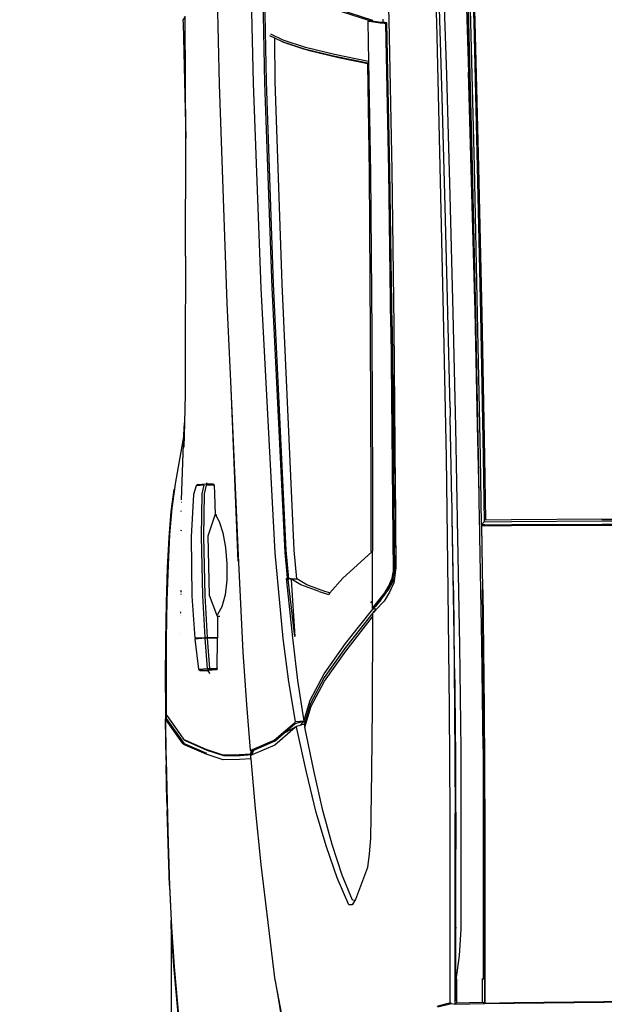
# Model space of a CAD drawing. Units: inches. Extents: x 0 to 4258, y 0 to 3769.
# Tile 8 of 30: x 3726 to 3749, y 3003 to 3042. Entities that reach past the tile are written whole.
import ezdxf

# ---------------------------------------------------------------- set-up
doc = ezdxf.new("R2010")
doc.units = ezdxf.units.IN
doc.header["$MEASUREMENT"] = 0
doc.layers.get('0').update_dxf_attribs({"color": 16})
doc.layers.add('A-ANNO-DIMS', color=250, linetype='Continuous', lineweight=18)
doc.layers.add('C-PKNG-VEHI', color=8, linetype='Continuous', lineweight=18)
doc.layers.add('Edges', color=250, linetype='Continuous')
doc.styles.get("Standard").update_dxf_attribs({"font": 'arial.ttf'})
doc.dimstyles.get("Standard").update_dxf_attribs({"dimtxt": 7, "dimasz": 0.18, "dimexe": 0.18, "dimexo": 0.0625, "dimgap": 0.09, "dimtad": 0, "dimtih": 1, "dimtoh": 1, "dimzin": 0, "dimdsep": 46, "dimlunit": 3, "dimtxsty": 'Standard', "dimcen": 0.09, "dimadec": 0, "dimazin": 0, "dimtfac": 1, "dimtofl": 0, "dimtmove": 0, "dimatfit": 3, "dimfxl": 1, "dimtolj": 1, "dimtzin": 0, "dimarcsym": 0})

# ---------------------------------------------------------------- blocks, each defined once
blk = doc.blocks.new('Nissan Qashqai pl')
at = {"layer": 'Edges'}
for p, q in [((10.4706, 11.5566), (10.4706, 12.2875)), ((10.4726, 11.5567), (10.4726, 12.2875)), ((10.4764, 11.5569), (10.4764, 12.2872)), ((10.4776, 11.5567), (10.4776, 12.2874)), ((11.056, 11.559), (11.0551, 11.7239)), ((11.0566, 11.5593), (11.0557, 11.724)), ((10.4769, 11.4474), (10.4764, 11.5569)), ((11.0572, 11.4499), (11.056, 11.559)), ((11.0579, 11.4504), (11.0566, 11.5593)), ((10.4706, 11.5566), (10.4711, 11.4469)), ((10.4731, 11.4469), (10.4726, 11.5567)), ((10.4781, 11.4469), (10.4776, 11.5567)), ((11.0579, 11.4146), (11.0572, 11.4499)), ((11.0585, 11.4142), (11.0579, 11.4504)), ((10.4711, 11.4469), (10.4715, 11.416)), ((10.4735, 11.414), (10.4731, 11.4469)), ((10.4773, 11.4146), (10.4769, 11.4474)), ((10.4785, 11.4111), (10.4781, 11.4469)), ((10.3947, 11.4148), (10.2218, 11.4114)), ((10.4715, 11.416), (10.3947, 11.4148)), ((10.3947, 11.4128), (10.4735, 11.414)), ((10.4773, 11.4107), (10.4735, 11.414)), ((10.4773, 11.4146), (10.4773, 11.4107)), ((10.6996, 11.4134), (10.5561, 11.4119)), ((10.5563, 11.4123), (10.6999, 11.4138)), ((10.7722, 11.4138), (10.6996, 11.4134)), ((10.6999, 11.4138), (10.7722, 11.4142)), ((10.7722, 11.4142), (10.7889, 11.4143)), ((10.7722, 11.4142), (10.7722, 11.4138)), ((10.7889, 11.4139), (10.7722, 11.4138)), ((10.7889, 11.4139), (10.7889, 11.4143)), ((10.7889, 11.4143), (10.7923, 11.4143)), ((10.7923, 11.4139), (10.7889, 11.4139)), ((10.7923, 11.4139), (10.7923, 11.4143)), ((10.7923, 11.4143), (10.7933, 11.4143)), ((10.7933, 11.4139), (10.7923, 11.4139)), ((10.7933, 11.4143), (10.827, 11.4145)), ((10.7933, 11.4139), (10.7933, 11.4143)), ((10.8267, 11.4141), (10.7933, 11.4139)), ((10.8267, 11.4141), (11.0585, 11.4142)), ((10.827, 11.4145), (11.0579, 11.4146)), ((11.0585, 11.4142), (11.0568, 11.4118)), ((11.0585, 11.4142), (11.0579, 11.4146)), ((11.0592, 11.3789), (11.0585, 11.4142)), ((9.8673, 11.4031), (9.701, 11.3983)), ((10.0431, 11.4075), (9.8673, 11.4031)), ((9.8673, 11.4012), (10.043, 11.4055)), ((10.0429, 11.4021), (9.8673, 11.3977)), ((10.2215, 11.406), (10.0429, 11.4021)), ((10.2216, 11.4037), (10.0429, 11.3998)), ((10.043, 11.4055), (10.2218, 11.4094)), ((10.2218, 11.4114), (10.0431, 11.4075)), ((10.2043, 11.4025), (10.0747, 11.3991)), ((10.0998, 11.3999), (10.2043, 11.4025)), ((10.2175, 11.4028), (10.2043, 11.4025)), ((10.3564, 11.406), (10.2175, 11.4028)), ((10.3945, 11.4094), (10.2215, 11.406)), ((10.3947, 11.4071), (10.2216, 11.4037)), ((10.2218, 11.4094), (10.3947, 11.4128)), ((10.4416, 11.4077), (10.3564, 11.406)), ((10.4773, 11.4107), (10.3945, 11.4094)), ((10.4416, 11.4078), (10.3947, 11.4071)), ((10.4519, 11.4079), (10.4416, 11.4077)), ((10.4519, 11.4079), (10.4416, 11.4078)), ((10.4416, 11.4077), (10.4416, 11.4078)), ((10.4524, 11.408), (10.4519, 11.4079)), ((10.4519, 11.4079), (10.4519, 11.4079)), ((10.4524, 11.4079), (10.4519, 11.4079)), ((10.4524, 11.4079), (10.4524, 11.408)), ((10.4533, 11.408), (10.4524, 11.408)), ((10.4533, 11.4079), (10.4524, 11.4079)), ((10.4638, 11.4081), (10.4533, 11.4079)), ((10.4638, 11.4081), (10.4533, 11.408)), ((10.4533, 11.4079), (10.4533, 11.408)), ((10.4914, 11.4087), (10.4638, 11.4081)), ((10.4773, 11.4107), (10.5561, 11.4119)), ((10.4773, 11.4107), (10.4785, 11.4111)), ((10.5563, 11.4123), (10.4785, 11.4111)), ((10.6223, 11.4109), (10.4914, 11.4087)), ((10.7493, 11.4125), (10.6223, 11.4109)), ((10.7493, 11.4125), (11.0294, 11.4126)), ((11.0294, 11.4118), (11.0281, 11.4118)), ((11.0294, 11.4125), (11.0294, 11.4126)), ((11.0295, 11.4116), (11.0294, 11.4118)), ((11.0568, 11.4118), (11.0294, 11.4118)), ((11.0574, 11.3804), (11.0568, 11.4118)), ((9.6472, 11.3861), (9.9278, 11.3949)), ((9.7011, 11.3963), (9.8673, 11.4012)), ((9.8673, 11.3977), (9.7014, 11.3929)), ((9.8673, 11.3954), (9.7014, 11.3906)), ((9.8565, 11.3931), (9.9794, 11.3967)), ((10.0429, 11.3998), (9.8673, 11.3954)), ((10.0747, 11.3991), (9.9278, 11.3949)), ((9.9794, 11.3967), (10.0965, 11.3998)), ((10.0965, 11.3998), (10.0998, 11.3999)), ((10.2201, 11.3759), (10.3586, 11.3791)), ((10.3586, 11.3791), (10.4931, 11.3817)), ((10.4931, 11.3817), (10.6237, 11.3839)), ((10.5566, 11.3765), (10.7, 11.378)), ((10.6649, 11.3783), (10.5576, 11.3766)), ((10.6649, 11.3783), (10.5866, 11.3772)), ((10.6237, 11.3839), (10.7502, 11.3855)), ((10.6908, 11.3785), (10.6649, 11.3783)), ((10.6649, 11.3783), (10.6772, 11.3784)), ((10.6966, 11.3787), (10.6772, 11.3784)), ((10.6772, 11.3784), (10.6908, 11.3785)), ((10.6991, 11.3786), (10.6908, 11.3785)), ((10.7144, 11.3788), (10.6966, 11.3787)), ((10.6999, 11.3786), (10.6991, 11.3786)), ((10.6999, 11.3786), (10.7808, 11.3793)), ((10.7144, 11.3788), (10.6999, 11.3786)), ((10.7, 11.378), (10.8279, 11.3787)), ((10.7239, 11.3789), (10.7144, 11.3788)), ((10.7248, 11.3789), (10.7239, 11.3789)), ((10.7808, 11.3793), (10.7248, 11.3789)), ((10.7502, 11.3855), (10.968, 11.3857)), ((10.7808, 11.3793), (10.8711, 11.3796)), ((10.9431, 11.3796), (10.8279, 11.3787)), ((10.8279, 11.3787), (11.0552, 11.3789)), ((10.9614, 11.3788), (10.8279, 11.3787)), ((10.896, 11.3796), (10.8711, 11.3796)), ((10.9097, 11.3796), (10.896, 11.3796)), ((10.9431, 11.3796), (10.9097, 11.3796)), ((10.9478, 11.3796), (10.9431, 11.3796)), ((10.9491, 11.3796), (10.9478, 11.3796)), ((10.9668, 11.3796), (10.9491, 11.3796)), ((10.9614, 11.3788), (10.9668, 11.3796)), ((10.9711, 11.3788), (10.9614, 11.3788)), ((10.9668, 11.3796), (10.967, 11.3796)), ((10.9765, 11.3796), (10.967, 11.3796)), ((10.968, 11.3857), (11, 11.3837)), ((10.9765, 11.3796), (10.9711, 11.3788)), ((10.9766, 11.3788), (10.9711, 11.3788)), ((10.9765, 11.3796), (10.9766, 11.3788)), ((10.9825, 11.3796), (10.9765, 11.3796)), ((11.0592, 11.3789), (10.9766, 11.3788)), ((11.0301, 11.3796), (10.9825, 11.3796)), ((11, 11.3837), (11.0301, 11.3796)), ((11.0287, 11.3804), (11.0301, 11.3804)), ((11.0301, 11.3803), (11.0292, 11.3802)), ((11.03, 11.3822), (11.03, 11.3824)), ((11.0301, 11.3803), (11.0301, 11.3804)), ((11.0301, 11.3804), (11.0554, 11.3804)), ((11.0554, 11.3804), (11.0301, 11.3803)), ((11.0301, 11.3796), (11.0301, 11.3803)), ((11.0554, 11.3804), (11.0574, 11.3804)), ((11.0592, 11.3789), (11.0574, 11.3804)), ((11.0582, 11.3742), (11.0592, 11.3789)), ((9.6514, 11.3592), (9.9312, 11.3681)), ((9.9312, 11.3681), (10.0776, 11.3722)), ((10.091, 11.3666), (9.9583, 11.363)), ((10.0776, 11.3722), (10.2201, 11.3759)), ((10.2191, 11.3699), (10.091, 11.3666)), ((10.2202, 11.3699), (10.2191, 11.3699)), ((10.2202, 11.3699), (10.2203, 11.3699)), ((10.3353, 11.3725), (10.2203, 11.3699)), ((10.3955, 11.368), (10.2211, 11.3646)), ((10.3353, 11.3725), (10.346, 11.3727)), ((10.4477, 11.3747), (10.346, 11.3727)), ((10.5572, 11.3704), (10.3955, 11.368)), ((10.4537, 11.3749), (10.4477, 11.3747)), ((10.4537, 11.3749), (10.4538, 11.3749)), ((10.4681, 11.3752), (10.4538, 11.3749)), ((10.4676, 11.3751), (10.4538, 11.3749)), ((10.5576, 11.3766), (10.4676, 11.3751)), ((10.5566, 11.3765), (10.4676, 11.3751)), ((10.4676, 11.3751), (10.4676, 11.3751)), ((10.5866, 11.3772), (10.4681, 11.3752)), ((10.7004, 11.372), (10.5572, 11.3704)), ((10.8279, 11.3727), (10.7004, 11.372)), ((11.0544, 11.3728), (10.8279, 11.3727)), ((11.0575, 11.3728), (11.0544, 11.3728)), ((11.0582, 11.3742), (11.0575, 11.3728)), ((11.0581, 11.3704), (11.0575, 11.3728)), ((11.0614, 11.3569), (11.0581, 11.3704)), ((11.0624, 11.3576), (11.0582, 11.3742)), ((9.9583, 11.363), (9.651, 11.3536)), ((9.8673, 11.3563), (9.7029, 11.3516)), ((10.0423, 11.3607), (9.8673, 11.3563)), ((10.2211, 11.3646), (10.0423, 11.3607)), ((10.2357, 11.3043), (10.53, 11.3068)), ((10.4182, 11.3058), (10.53, 11.3068)), ((10.53, 11.3068), (10.5301, 11.3068)), ((10.5301, 11.3068), (10.5323, 11.3065)), ((10.5323, 11.3065), (10.5419, 11.3051)), ((9.696, 11.2932), (9.8644, 11.2982)), ((9.8644, 11.2982), (10.0472, 11.3018)), ((9.8681, 11.2959), (9.8678, 11.2935)), ((10.0476, 11.2996), (9.8681, 11.2959)), ((9.8681, 11.2959), (9.869, 11.2946)), ((9.869, 11.2946), (9.8689, 11.2927)), ((10.0477, 11.2982), (9.869, 11.2946)), ((10.0472, 11.3018), (10.2357, 11.3043)), ((10.2367, 11.3022), (10.0476, 11.2996)), ((10.2369, 11.3008), (10.0477, 11.2982)), ((10.2367, 11.3022), (10.5351, 11.305)), ((10.2369, 11.3008), (10.5348, 11.3036)), ((10.4153, 11.3058), (10.2954, 11.3046)), ((10.4153, 11.3058), (10.4174, 11.3058)), ((10.4174, 11.3058), (10.4181, 11.3058)), ((10.4181, 11.3058), (10.4182, 11.3058)), ((10.5422, 11.3021), (10.5348, 11.3036)), ((10.5424, 11.3035), (10.5351, 11.305)), ((10.5366, 11.3048), (10.536, 11.305)), ((10.5379, 11.3052), (10.5381, 11.305)), ((10.5419, 11.3051), (10.5463, 11.3031)), ((10.5419, 11.3051), (10.5479, 11.3042)), ((10.5522, 11.2977), (10.5422, 11.3021)), ((10.5472, 11.3014), (10.5424, 11.3035)), ((10.5463, 11.3031), (10.5551, 11.2984)), ((10.5546, 11.2982), (10.5472, 11.3014)), ((10.5479, 11.3042), (10.5589, 11.2991)), ((10.5598, 11.2935), (10.5522, 11.2977)), ((10.5583, 11.296), (10.5546, 11.2982)), ((10.5551, 11.2984), (10.5583, 11.296)), ((10.5612, 11.2944), (10.5583, 11.296)), ((10.5589, 11.2991), (10.57, 11.2925)), ((10.5683, 11.2885), (10.5612, 11.2944)), ((9.8637, 11.291), (9.8643, 11.291)), ((9.8643, 11.291), (9.8677, 11.291)), ((9.8675, 11.2887), (9.8655, 11.2754)), ((9.8686, 11.2879), (9.8665, 11.2747)), ((9.8677, 11.291), (9.8675, 11.2887)), ((9.8678, 11.2935), (9.8677, 11.291)), ((9.8689, 11.2927), (9.8686, 11.2879)), ((10.5764, 11.28), (10.5598, 11.2935)), ((10.5683, 11.2885), (10.573, 11.285)), ((10.575, 11.2829), (10.5683, 11.2885)), ((10.57, 11.2925), (10.5811, 11.2822)), ((10.573, 11.285), (10.5769, 11.2818)), ((10.5776, 11.2808), (10.575, 11.2829)), ((10.5796, 11.2824), (10.5796, 11.2787)), ((10.5811, 11.2822), (10.5821, 11.2808)), ((10.5811, 11.2822), (10.5834, 11.28)), ((9.8652, 11.2788), (9.8516, 11.2363)), ((9.8652, 11.2738), (9.8516, 11.2313)), ((9.8652, 11.2738), (9.8652, 11.2788)), ((9.8655, 11.2754), (9.8652, 11.2738)), ((9.8652, 11.2735), (9.8665, 11.2747)), ((9.8652, 11.2738), (9.8652, 11.2738)), ((9.8652, 11.2738), (9.8652, 11.2735)), ((9.8652, 11.2735), (9.8664, 11.2728)), ((9.8665, 11.2747), (9.8664, 11.2728)), ((9.8664, 11.2728), (9.9149, 11.2736)), ((9.9149, 11.2736), (9.9066, 11.2322)), ((9.9169, 11.2728), (9.9086, 11.2313)), ((9.9177, 11.2728), (9.9106, 11.2373)), ((9.9149, 11.2736), (10.0505, 11.276)), ((9.9177, 11.2728), (9.9169, 11.2728)), ((10.0501, 11.2747), (9.9177, 11.2728)), ((10.2453, 11.2762), (10.0501, 11.2747)), ((10.0505, 11.276), (10.2453, 11.2777)), ((10.2453, 11.2777), (10.4289, 11.2783)), ((10.4292, 11.2767), (10.2453, 11.2762)), ((10.4289, 11.2783), (10.5092, 11.2783)), ((10.5099, 11.2768), (10.4292, 11.2767)), ((10.5099, 11.2768), (10.5092, 11.2783)), ((10.5092, 11.2783), (10.5094, 11.2783)), ((10.5094, 11.2783), (10.51, 11.2776)), ((10.5783, 11.2783), (10.5094, 11.2783)), ((10.51, 11.2776), (10.5099, 11.2768)), ((10.51, 11.2776), (10.5419, 11.2423)), ((10.5705, 11.2771), (10.5709, 11.2767)), ((10.5709, 11.2767), (10.5719, 11.2759)), ((10.5783, 11.2783), (10.5764, 11.28)), ((10.5796, 11.2787), (10.5776, 11.2808)), ((10.5776, 11.2808), (10.5783, 11.2783)), ((10.5796, 11.2787), (10.5783, 11.2783)), ((10.6215, 11.2456), (10.5796, 11.2787)), ((10.5821, 11.2808), (10.5834, 11.2793)), ((10.5825, 11.2806), (10.5834, 11.2793)), ((10.5834, 11.28), (10.5851, 11.2783)), ((10.5834, 11.2793), (10.5835, 11.2793)), ((10.5835, 11.2793), (10.584, 11.2787)), ((10.584, 11.2789), (10.584, 11.2793)), ((10.584, 11.2787), (10.584, 11.2789)), ((10.584, 11.2787), (10.6261, 11.2458)), ((10.584, 11.2787), (10.5851, 11.2783)), ((10.5843, 11.2787), (10.584, 11.2787)), ((10.5847, 11.2787), (10.5843, 11.2787)), ((10.5851, 11.2783), (10.5892, 11.2783)), ((10.6306, 11.2459), (10.5892, 11.2783)), ((10.5892, 11.2783), (10.6988, 11.2779)), ((10.6988, 11.2779), (10.7769, 11.2774)), ((10.7769, 11.2774), (10.858, 11.2759)), ((10.858, 11.2759), (10.8766, 11.2745)), ((10.8766, 11.2745), (10.8932, 11.2722)), ((10.8932, 11.2722), (10.932, 11.258)), ((10.932, 11.258), (10.9335, 11.257)), ((10.933, 11.2541), (10.9026, 11.2417)), ((10.9384, 11.2497), (10.9059, 11.2355)), ((10.9335, 11.257), (10.933, 11.2541)), ((10.9335, 11.257), (10.9386, 11.2537)), ((10.9386, 11.2537), (10.9384, 11.2497)), ((9.9106, 11.2373), (9.9018, 11.2021)), ((10.5419, 11.2423), (10.56, 11.2265)), ((10.6583, 11.2197), (10.6215, 11.2456)), ((10.6261, 11.2458), (10.6627, 11.22)), ((10.6671, 11.2203), (10.6306, 11.2459)), ((10.9026, 11.2417), (10.8653, 11.2297)), ((10.9059, 11.2355), (10.8682, 11.2226)), ((9.9066, 11.2322), (9.8978, 11.197)), ((9.9086, 11.2313), (9.8998, 11.196)), ((10.56, 11.2265), (10.5584, 11.2206)), ((10.5584, 11.2136), (10.5617, 11.2251)), ((10.56, 11.2265), (10.5617, 11.2251)), ((10.8653, 11.2297), (10.8239, 11.2181)), ((10.8682, 11.2226), (10.8264, 11.21)), ((10.5584, 11.2206), (10.5502, 11.1986)), ((10.5584, 11.2136), (10.5502, 11.1916)), ((10.69, 11.2028), (10.6583, 11.2197)), ((10.6627, 11.22), (10.6943, 11.2032)), ((10.6976, 11.2041), (10.6671, 11.2203)), ((10.8239, 11.2181), (10.7754, 11.2071)), ((9.9018, 11.2021), (9.8931, 11.1752)), ((10.5502, 11.1986), (10.543, 11.1865)), ((10.7155, 11.1952), (10.69, 11.2028)), ((10.6943, 11.2032), (10.7155, 11.1969)), ((10.7228, 11.1965), (10.6976, 11.2041)), ((10.7754, 11.2071), (10.7228, 11.1965)), ((10.8264, 11.21), (10.7776, 11.1982)), ((9.8978, 11.197), (9.8891, 11.1701)), ((9.8911, 11.1693), (9.8998, 11.196)), ((10.543, 11.1865), (10.5079, 11.1835)), ((10.5502, 11.1916), (10.543, 11.1795)), ((10.543, 11.1795), (10.543, 11.1865)), ((10.6144, 11.1813), (10.6664, 11.1875)), ((10.6664, 11.1875), (10.7155, 11.1952)), ((10.7155, 11.1957), (10.7155, 11.1969)), ((10.7155, 11.1969), (10.7192, 11.1957)), ((10.7209, 11.1902), (10.7155, 11.1957)), ((10.7155, 11.1952), (10.7155, 11.1957)), ((10.7186, 11.1848), (10.7155, 11.1952)), ((10.7155, 11.1952), (10.7165, 11.1851)), ((10.7192, 11.1957), (10.7228, 11.1965)), ((10.7192, 11.1957), (10.7209, 11.1902)), ((10.7209, 11.1902), (10.7221, 11.1861)), ((10.7247, 11.1867), (10.7222, 11.186)), ((10.7776, 11.1982), (10.7247, 11.1867)), ((9.8931, 11.1751), (9.8911, 11.1693)), ((9.8931, 11.1751), (9.8931, 11.1752)), ((10.5079, 11.1835), (10.1849, 11.1687)), ((10.543, 11.1771), (10.5079, 11.1739)), ((10.5109, 11.1721), (10.5417, 11.1748)), ((10.543, 11.1771), (10.5417, 11.1748)), ((10.5417, 11.1748), (10.5427, 11.1739)), ((10.5436, 11.1754), (10.5427, 11.1739)), ((10.5439, 11.1796), (10.543, 11.1795)), ((10.543, 11.1795), (10.543, 11.1771)), ((10.544, 11.1763), (10.543, 11.1771)), ((10.544, 11.1763), (10.5436, 11.1754)), ((10.5439, 11.1796), (10.613, 11.1841)), ((10.547, 11.1767), (10.544, 11.1763)), ((10.5458, 11.1742), (10.6144, 11.1813)), ((10.613, 11.1841), (10.547, 11.1767)), ((10.6678, 11.177), (10.6152, 11.1702)), ((10.7137, 11.1846), (10.6678, 11.177)), ((10.7165, 11.1851), (10.7137, 11.1846)), ((10.7177, 11.1838), (10.7165, 11.1851)), ((10.7387, 11.1593), (10.7177, 11.1838)), ((10.7312, 11.1701), (10.7186, 11.1848)), ((10.7221, 11.1861), (10.7222, 11.1859)), ((10.7222, 11.186), (10.7221, 11.1861)), ((10.7222, 11.186), (10.7222, 11.1859)), ((10.7222, 11.1859), (10.7232, 11.1848)), ((10.7222, 11.1859), (10.7224, 11.1855)), ((10.7224, 11.1855), (10.7312, 11.1701)), ((10.7232, 11.1848), (10.7228, 11.1859)), ((10.7232, 11.1848), (10.7449, 11.1598)), ((10.7257, 11.1853), (10.7256, 11.1854)), ((11.0357, 11.1613), (11.1598, 11.1847)), ((11.0492, 11.1635), (11.1336, 11.1772)), ((9.8891, 11.1701), (9.8818, 11.1551)), ((9.8911, 11.1691), (9.8867, 11.16)), ((9.8911, 11.1693), (9.8911, 11.1691)), ((10.1849, 11.1687), (9.9393, 11.1602)), ((10.5079, 11.1739), (10.1849, 11.1585)), ((10.1894, 11.1563), (10.5109, 11.1721)), ((10.6152, 11.1702), (10.5113, 11.1603)), ((10.5427, 11.1739), (10.5458, 11.1742)), ((10.7397, 11.1602), (10.7312, 11.1701)), ((11.0357, 11.1613), (11.0491, 11.1635)), ((11.0492, 11.1635), (11.0491, 11.1635)), ((9.8867, 11.16), (9.8838, 11.1541)), ((9.9393, 11.1602), (9.8867, 11.16)), ((10.1849, 11.1585), (9.9393, 11.1497)), ((9.9411, 11.1475), (10.1894, 11.1563)), ((10.5113, 11.1603), (10.19, 11.1433)), ((10.7501, 11.1327), (10.7387, 11.1593)), ((10.7507, 11.1344), (10.7397, 11.1602)), ((10.7449, 11.1598), (10.7563, 11.1333)), ((11.0304, 11.1603), (10.8896, 11.1434)), ((11.0304, 11.1603), (11.0357, 11.1613)), ((9.8101, 11.1449), (9.9411, 11.1475)), ((9.9393, 11.1497), (9.8119, 11.1472)), ((10.19, 11.1433), (9.9414, 11.1341)), ((10.8896, 11.1434), (10.8218, 11.1365)), ((9.9414, 11.1341), (9.8143, 11.1312)), ((10.6955, 11.1257), (10.7509, 11.1302)), ((10.7507, 11.1309), (10.7501, 11.1327)), ((10.7511, 11.1335), (10.7507, 11.1344)), ((10.7507, 11.1344), (10.7524, 11.1335)), ((10.751, 11.131), (10.7507, 11.1309)), ((10.7509, 11.1302), (10.7507, 11.1309)), ((10.7522, 11.1311), (10.7509, 11.1302)), ((10.7516, 11.131), (10.7509, 11.1302)), ((10.7519, 11.1314), (10.7511, 11.1335)), ((10.7519, 11.1314), (10.7516, 11.131)), ((10.7522, 11.1311), (10.7516, 11.131)), ((10.7526, 11.1318), (10.7519, 11.1314)), ((10.7553, 11.1307), (10.7522, 11.1311)), ((10.7524, 11.1335), (10.7526, 11.1318)), ((10.7524, 11.1335), (10.7556, 11.1319)), ((10.7532, 11.1321), (10.7526, 11.1318)), ((10.7526, 11.1318), (10.7526, 11.1314)), ((10.7556, 11.1319), (10.7532, 11.1321)), ((10.7563, 11.1169), (10.7553, 11.1307)), ((10.7556, 11.1319), (10.7561, 11.1317)), ((10.7563, 11.1319), (10.7561, 11.1319)), ((10.7563, 11.1315), (10.7561, 11.1317)), ((10.7561, 11.1317), (10.7563, 11.1317)), ((10.7563, 11.1333), (10.7569, 11.1317)), ((10.7563, 11.1317), (10.7563, 11.1319)), ((10.7563, 11.1317), (10.7569, 11.1317)), ((10.7569, 11.1316), (10.7563, 11.1317)), ((10.7563, 11.1315), (10.7563, 11.1317)), ((10.7572, 11.1178), (10.7563, 11.1315)), ((10.7573, 11.1307), (10.7563, 11.1315)), ((10.7569, 11.1317), (10.7569, 11.1316)), ((10.7569, 11.1316), (10.7573, 11.1307)), ((10.7604, 11.131), (10.7573, 11.1307)), ((10.7615, 11.1311), (10.7604, 11.131)), ((10.8218, 11.1365), (10.7615, 11.1311)), ((10.7615, 11.1311), (10.7623, 11.1173)), ((10.312, 11.1064), (10.5147, 11.1156)), ((10.312, 11.1064), (10.5214, 11.1149)), ((10.5147, 11.1156), (10.6318, 11.1213)), ((10.6318, 11.1213), (10.6955, 11.1257)), ((10.7565, 11.0969), (10.7563, 11.1169)), ((10.7575, 11.0979), (10.7572, 11.1178)), ((10.7623, 11.1173), (10.7626, 11.0974)), ((10.2081, 11.1017), (10.312, 11.1064)), ((9.8024, 11.0892), (9.9426, 11.0923)), ((9.9426, 11.0923), (10.2081, 11.1017)), ((10.4653, 11.0881), (10.4732, 11.0925)), ((10.4732, 11.0925), (10.4871, 11.0967)), ((10.4871, 11.0967), (10.5048, 11.1002)), ((10.5048, 11.1002), (10.5246, 11.1019)), ((10.5246, 11.1019), (10.5445, 11.1017)), ((10.5445, 11.1017), (10.5625, 11.0996)), ((10.5625, 11.0996), (10.5769, 11.0957)), ((10.5769, 11.0957), (10.5863, 11.0904)), ((10.5885, 11.0931), (10.5885, 11.0904)), ((10.7497, 11.0763), (10.7565, 11.0969)), ((10.7507, 11.0773), (10.7575, 11.0979)), ((10.7626, 11.0974), (10.7559, 11.0767)), ((10.4274, 11.0767), (10.4275, 11.0856)), ((10.4275, 11.0856), (10.4293, 11.0863)), ((10.4293, 11.0863), (10.4291, 11.0765)), ((10.4293, 11.0863), (10.4398, 11.0868)), ((10.4398, 11.0868), (10.4653, 11.0878)), ((10.4653, 11.0881), (10.4652, 11.0897)), ((10.4653, 11.0877), (10.4653, 11.0881)), ((10.4653, 11.0878), (10.4653, 11.0881)), ((10.4653, 11.0881), (10.4653, 11.0881)), ((10.4653, 11.0877), (10.4653, 11.0878)), ((10.4908, 11.0793), (10.4653, 11.0877)), ((10.563, 11.0809), (10.4908, 11.0793)), ((10.5867, 11.0897), (10.563, 11.0809)), ((10.5863, 11.0904), (10.5867, 11.0897)), ((10.5885, 11.0904), (10.5867, 11.0897)), ((10.5885, 11.0904), (10.6141, 11.0905)), ((10.6141, 11.0905), (10.615, 11.0905)), ((10.6142, 11.0782), (10.6141, 11.0905)), ((10.6517, 11.0902), (10.615, 11.0905)), ((10.615, 11.0905), (10.6151, 11.0782)), ((10.6151, 11.078), (10.6518, 11.0808)), ((10.6518, 11.0808), (10.6517, 11.0902)), ((10.6517, 11.0902), (10.6535, 11.0895)), ((10.6518, 11.0784), (10.6518, 11.0808)), ((10.6518, 11.0808), (10.6536, 11.0803)), ((10.6536, 11.0803), (10.6518, 11.0784)), ((10.6535, 11.0895), (10.6543, 11.0786)), ((10.6535, 11.0895), (10.6536, 11.0803)), ((10.6536, 11.0803), (10.6537, 11.0783)), ((10.6578, 11.0814), (10.6543, 11.0786)), ((10.4263, 11.0777), (10.4274, 11.0767)), ((10.4274, 11.0762), (10.4274, 11.0767)), ((10.4282, 11.0666), (10.4274, 11.0762)), ((10.4291, 11.0765), (10.4398, 11.0741)), ((10.4398, 11.0718), (10.4291, 11.0741)), ((10.4291, 11.0741), (10.4299, 11.0644)), ((10.4398, 11.0741), (10.4909, 11.0734)), ((10.4909, 11.0711), (10.4398, 11.0718)), ((10.4909, 11.0734), (10.563, 11.075)), ((10.5631, 11.0727), (10.4909, 11.0711)), ((10.563, 11.075), (10.6142, 11.0779)), ((10.6142, 11.0756), (10.5631, 11.0727)), ((10.6142, 11.0779), (10.6142, 11.0782)), ((10.6142, 11.0765), (10.6142, 11.0779)), ((10.615, 11.0765), (10.6142, 11.0765)), ((10.6142, 11.0756), (10.6142, 11.0765)), ((10.615, 11.0639), (10.6142, 11.0756)), ((10.6151, 11.0765), (10.615, 11.0765)), ((10.615, 11.0765), (10.6151, 11.0639)), ((10.6518, 11.0784), (10.6151, 11.0756)), ((10.6151, 11.0782), (10.6151, 11.078)), ((10.6151, 11.078), (10.6151, 11.0765)), ((10.6151, 11.0765), (10.6151, 11.0756)), ((10.6151, 11.0756), (10.616, 11.0629)), ((10.616, 11.0629), (10.6526, 11.0674)), ((10.6526, 11.0674), (10.6518, 11.0784)), ((10.6526, 11.0674), (10.6543, 11.0693)), ((10.6543, 11.0786), (10.6537, 11.0783)), ((10.6537, 11.0783), (10.6543, 11.0693)), ((10.6543, 11.0693), (10.6543, 11.0786)), ((10.7385, 11.051), (10.7497, 11.0763)), ((10.7396, 11.0519), (10.7507, 11.0773)), ((10.7549, 11.0776), (10.743, 11.0503)), ((10.7559, 11.0767), (10.7448, 11.0511)), ((10.4282, 11.0666), (10.4299, 11.0644)), ((10.4299, 11.0644), (10.4406, 11.0612)), ((10.4406, 11.0612), (10.4919, 11.0584)), ((10.4919, 11.0584), (10.564, 11.0591)), ((10.564, 11.0591), (10.6151, 11.0628)), ((10.6151, 11.0639), (10.615, 11.0639)), ((10.6151, 11.0628), (10.615, 11.0639)), ((10.6151, 11.0639), (10.6151, 11.0628)), ((9.8643, 11.0514), (9.8598, 11.0514)), ((9.8614, 11.0504), (9.8647, 11.0485)), ((10.0085, 11.0519), (9.8643, 11.0514)), ((9.8647, 11.0485), (9.869, 11.0488)), ((9.869, 11.0488), (10.0085, 11.0519)), ((10.0124, 11.0519), (10.0085, 11.0519)), ((10.1513, 11.0517), (10.0124, 11.0519)), ((10.1513, 11.0517), (10.2677, 11.0512)), ((10.2677, 11.0512), (10.3189, 11.0511)), ((10.3189, 11.0511), (10.3537, 11.0503)), ((10.3537, 11.0503), (10.3832, 11.0496)), ((10.3679, 11.0497), (10.3537, 11.0503)), ((10.3679, 11.0497), (10.4275, 11.0391)), ((10.4468, 11.0466), (10.3679, 11.0497)), ((10.4502, 11.0466), (10.4503, 11.0465)), ((10.4613, 11.0464), (10.4603, 11.0465)), ((10.4838, 11.0465), (10.4852, 11.046)), ((10.5565, 11.0456), (10.5591, 11.0464)), ((10.5615, 11.0464), (10.5617, 11.0457)), ((10.583, 11.0457), (10.5835, 11.0461)), ((10.5836, 11.0461), (10.5832, 11.0457)), ((10.5847, 11.0461), (10.5841, 11.0457)), ((10.5873, 11.0461), (10.5873, 11.0461)), ((10.6087, 11.0458), (10.6087, 11.0458)), ((10.7087, 11.0289), (10.7363, 11.0483)), ((10.7424, 11.0499), (10.7125, 11.0285)), ((10.7429, 11.0485), (10.7148, 11.0284)), ((10.7363, 11.0483), (10.7376, 11.0492)), ((10.7387, 11.0502), (10.7376, 11.0492)), ((10.7376, 11.0492), (10.7378, 11.0495)), ((10.7378, 11.0495), (10.7385, 11.051)), ((10.7378, 11.0495), (10.7379, 11.0496)), ((10.7387, 11.0502), (10.7396, 11.0519)), ((10.7424, 11.0499), (10.743, 11.0503)), ((10.7429, 11.0488), (10.7432, 11.0488)), ((10.7432, 11.0488), (10.7429, 11.0485)), ((10.744, 11.0494), (10.7432, 11.0488)), ((10.7448, 11.0511), (10.744, 11.0494)), ((11.0798, 11.0434), (11.0576, 11.0416)), ((11.059, 11.0419), (11.0768, 11.0434)), ((10.4275, 11.0391), (10.4304, 11.0385)), ((10.4304, 11.0385), (10.4339, 11.0381)), ((10.4345, 11.0379), (10.4339, 11.0381)), ((10.4339, 11.0381), (10.4573, 11.0349)), ((10.4613, 11.0343), (10.4345, 11.0379)), ((10.4573, 11.0349), (10.4889, 11.0323)), ((10.4926, 11.0317), (10.4613, 11.0343)), ((10.4889, 11.0323), (10.526, 11.0304)), ((10.5294, 11.0298), (10.4926, 11.0317)), ((10.9152, 11.0321), (10.8642, 11.0304)), ((10.8642, 11.0305), (10.8759, 11.031)), ((10.8644, 11.0306), (10.8759, 11.031)), ((10.8759, 11.031), (10.9158, 11.0324)), ((10.9152, 11.0321), (10.9577, 11.0341)), ((10.9158, 11.0324), (10.9657, 11.0347)), ((10.9649, 11.0344), (10.9577, 11.0341)), ((10.9577, 11.0341), (11.1283, 11.0341)), ((11.0127, 11.0375), (10.9649, 11.0344)), ((10.9657, 11.0347), (11.0138, 11.0377)), ((11.0576, 11.0416), (11.0127, 11.0375)), ((11.0138, 11.0377), (11.059, 11.0419)), ((10.526, 11.0304), (10.569, 11.0291)), ((10.5719, 11.0285), (10.5294, 11.0298)), ((10.569, 11.0291), (10.5919, 11.0287)), ((10.6176, 11.0277), (10.5719, 11.0285)), ((10.5919, 11.0287), (10.5936, 11.0286)), ((10.5936, 11.0286), (10.6151, 11.0283)), ((10.6151, 11.0283), (10.6644, 11.028)), ((10.6651, 11.0274), (10.6176, 11.0277)), ((10.6644, 11.028), (10.7078, 11.0282)), ((10.677, 11.0275), (10.6651, 11.0274)), ((10.7082, 11.0285), (10.6729, 11.0284)), ((10.68, 11.0274), (10.677, 11.0275)), ((10.6809, 11.0274), (10.68, 11.0274)), ((10.6809, 11.0274), (10.7128, 11.0275)), ((10.7078, 11.0282), (10.7083, 11.0285)), ((10.7082, 11.0285), (10.7078, 11.0282)), ((10.7085, 11.0289), (10.7082, 11.0285)), ((10.7083, 11.0285), (10.7082, 11.0285)), ((10.7083, 11.0285), (10.7087, 11.0289)), ((10.7125, 11.0285), (10.7083, 11.0285)), ((10.7146, 11.0286), (10.7125, 11.0285)), ((10.7125, 11.0285), (10.7139, 11.0278)), ((10.7134, 11.0275), (10.7128, 11.0275)), ((10.7625, 11.0281), (10.7134, 11.0275)), ((10.724, 11.0275), (10.7134, 11.0275)), ((10.7148, 11.0284), (10.7139, 11.0278)), ((10.7628, 11.0283), (10.7139, 11.0278)), ((10.724, 11.0275), (10.7685, 11.0281)), ((10.7628, 11.0281), (10.7625, 11.0281)), ((10.7628, 11.0283), (10.8131, 11.0292)), ((10.7628, 11.0281), (10.8131, 11.029)), ((10.7688, 11.0281), (10.7685, 11.0281)), ((10.8131, 11.029), (10.7688, 11.0281)), ((10.8131, 11.0292), (10.8644, 11.0306)), ((10.8132, 11.029), (10.8131, 11.029)), ((10.8132, 11.029), (10.8139, 11.029)), ((10.8142, 11.029), (10.8139, 11.029)), ((10.8142, 11.029), (10.8241, 11.0293)), ((10.8142, 11.029), (10.8142, 11.029)), ((10.8242, 11.0293), (10.8241, 11.0293)), ((10.8246, 11.0293), (10.8242, 11.0293)), ((10.8642, 11.0304), (10.8246, 11.0293))]:
    blk.add_line(p, q, dxfattribs=at)
blk = doc.blocks.new('car')
blk.add_blockref('Nissan Qashqai pl', (-9.7433, -11.9151))
blk = doc.blocks.new('*D66')
at = {"layer": 'A-ANNO-DIMS', "color": 0, "lineweight": -2, "transparency": 16777216}
for p, q in [((3725.517, 3125.846), (3703.936, 3125.846)), ((3704.116, 3125.666), (3704.116, 3058.01)), ((3704.116, 2982.935), (3704.116, 3050.591)), ((3725.517, 2982.755), (3703.936, 2982.755))]:
    blk.add_line(p, q, dxfattribs=at)
at = {"layer": 'A-ANNO-DIMS', "color": 0, "transparency": 16777216}
for points in [[(3704.086, 3125.666), (3704.146, 3125.666), (3704.116, 3125.846)], [(3704.086, 2982.935), (3704.146, 2982.935), (3704.116, 2982.755)]]:
    blk.add_solid(points, dxfattribs=at)
at = {"layer": 'Defpoints', "color": 0, "transparency": 16777216}
for p in [(3725.58, 3125.846), (3704.116, 2982.755), (3725.58, 2982.755)]:
    blk.add_point(p, dxfattribs=at)
at = {"layer": 'A-ANNO-DIMS', "color": 0, "transparency": 16777216, "insert": (3704.116, 3054.301), "char_height": 7, "attachment_point": 5}
blk.add_mtext('\\A1;CAR 11\'-11"', dxfattribs=at)

msp = doc.modelspace()

# ---------------------------------------------------------------- block references
at = {"layer": 'C-PKNG-VEHI', "xscale": 32.66500240257601, "yscale": 32.66500240257601, "zscale": 32.66500240257601, "rotation": 270}
msp.add_blockref('car', (3760.419, 3045.57), dxfattribs=at)

# ---------------------------------------------------------------- dimensions: what is measured, and where the dimension line sits
at = {"layer": 'A-ANNO-DIMS'}
dim = msp.add_linear_dim(base=(3704.116, 2982.755), p1=(3725.58, 3125.846), p2=(3725.58, 2982.755), angle=270, text='CAR <>', dimstyle='Standard', override={"dimdec": 1, "dimlfac": 1, "dimrnd": 0, "dimzin": 1, "dimdsep": 46, "dimlunit": 4, "dimfrac": 2}, dxfattribs=at)
dim.commit()
dim.dimension.update_dxf_attribs({"geometry": '*D66', "text_midpoint": (3704.116, 3054.301)})

doc.saveas('drawing.dxf')
